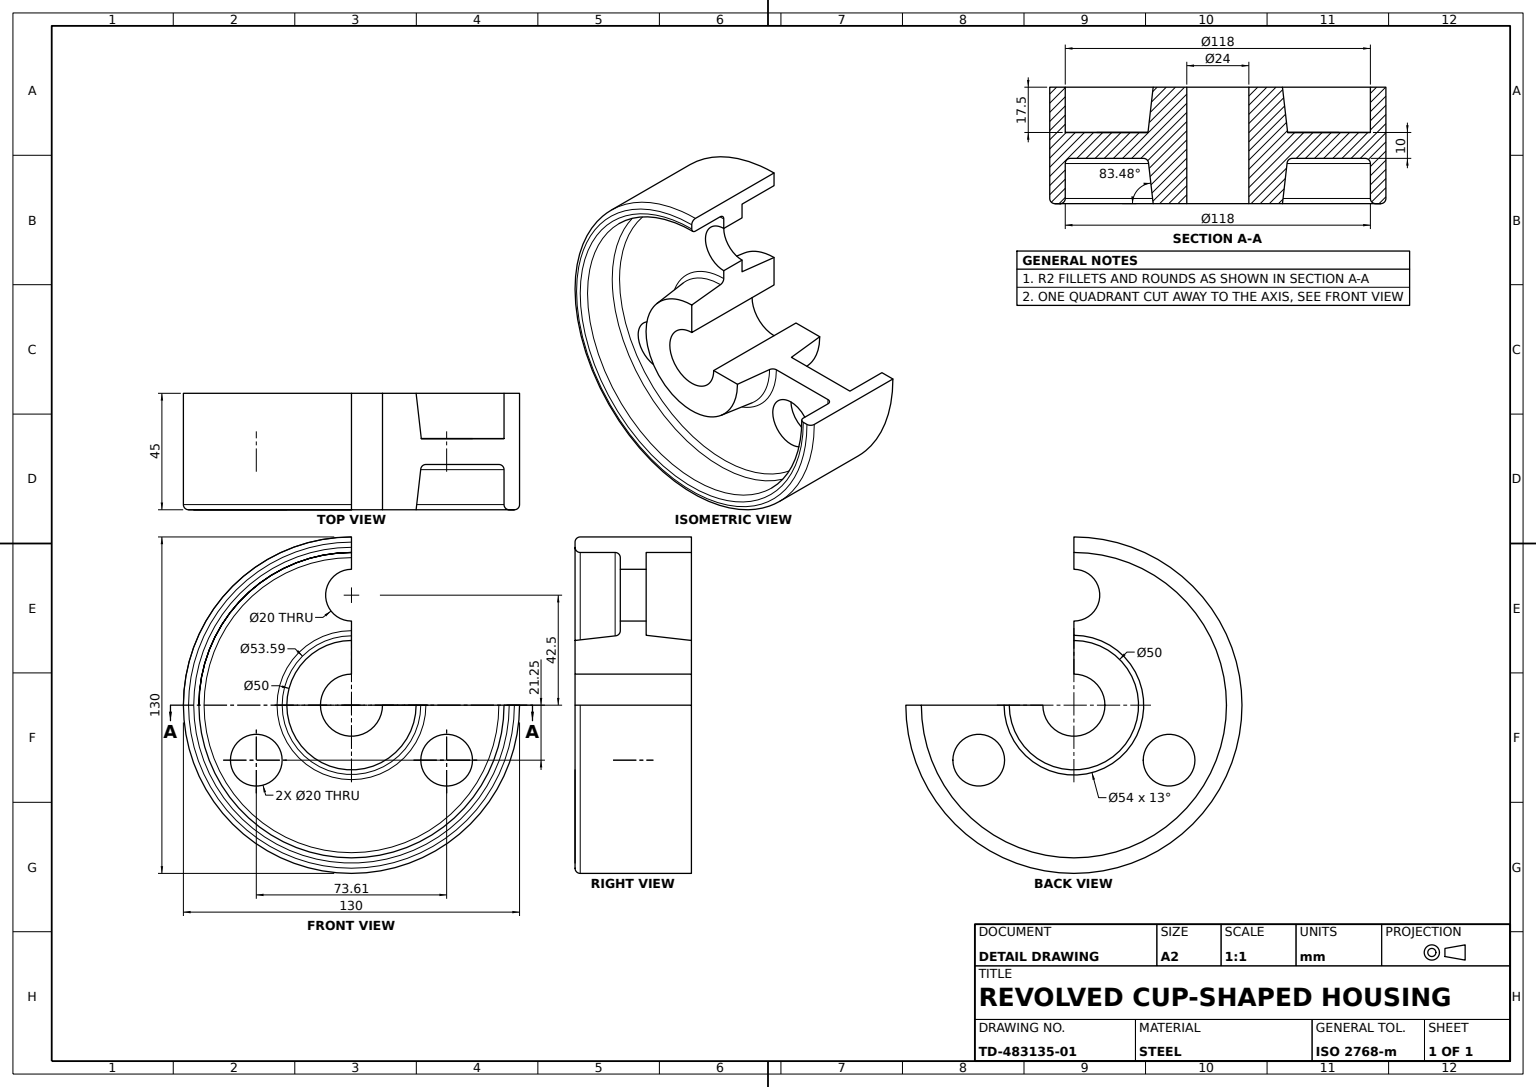
SolidWorks part; units mm, degrees
material "Plain Carbon Steel"
ref_plane "Front Plane" through (0, 0, 0) normal (0, 0, 1) x (1, 0, 0)
ref_plane "Top Plane" through (0, 0, 0) normal (0, 1, 0) x (1, 0, 0)
ref_plane "Right Plane" through (0, 0, 0) normal (1, 0, 0) x (0, 0, -1)
sketch "Wheel Profile Sketch" plane through (0, 0, 0) normal (0, 0, 1) x (1, 0, 0)
  line L0 (-53.0847, 0) -> (60.8825, 0)
  line L1 (0, 50.2951) -> (0, -47.8033) construction
  line L2 (0, 0) -> (0, 12)
  line L3 (22.5, 12) -> (-22.5, 12)
  line L4 (-22.5, 12) -> (-22.5, 25)
  line L5 (-22.5, 25) -> (-5, 27)
  line L6 (-5, 27) -> (-5, 59)
  line L7 (-5, 59) -> (-22.5, 59)
  line L8 (-22.5, 59) -> (-22.5, 65)
  line L9 (-22.5, 65) -> (22.5, 65)
  line L10 (22.5, 59) -> (22.5, 65)
  line L11 (5, 59) -> (22.5, 59)
  line L12 (5, 27) -> (5, 59)
  line L13 (22.5, 25) -> (5, 27)
  line L14 (22.5, 12) -> (22.5, 25)
  point P15 (0, 65)
  dimension "D1" = 12
  dimension "D2" = 22.5
  dimension "D3" = 13
  dimension "D4" = 15
  dimension "D5" = 6
  dimension "D6" = 5
  dimension "D7" = 53
  dimension "D8" = 17.5
  dimension "D9" = 53.0847
  dimension "D10" = 113.9672
revolve "Wheel Body Revolve" add sketch "Wheel Profile Sketch" angle 360 about L0
sketch "Rim Slot Sketch" plane through (5, 0, 0) normal (1, 0, 0) x (0, 0, -1)
  circle A0 centre (0, 0) radius 42.5 construction
  circle A1 centre (0, 42.5) radius 10
  circle A2 centre (36.8061, -21.25) radius 10
  circle A3 centre (-36.8061, -21.25) radius 10
  point P12 (0, 0)
  dimension "D1" = 85
  dimension "D2" = 20
  dimension "D4" = 63.75
  dimension "D3" = 3
extrude "Rim Slot Cut" cut sketch "Rim Slot Sketch" against normal through all contours A1 | A3 | A2
fillet "Edge Fillet R2 A" radius 2 3 edges at (5, 0, 59) (5, 0, 27) (22.5, 0, 65)
fillet "Edge Fillet R2 B" radius 2 1 edges at (22.5, 0, 59)
sketch "Web Relief Sketch" plane through (5, 0, 0) normal (1, 0, 0) x (0, 0, -1)
  line L0 (0, 77.9926) -> (0, 0)
  line L1 (0, 0) -> (85.2806, 0)
  arc A0 (0, 77.9926) -> (85.2806, 0) centre (13.9611, 7.6372) cw
  circle A1 centre (0, 42.5) radius 10 construction
  dimension "D1" = 71.7273
  dimension "D2" = 13.9611
  dimension "D3" = 85.2806
extrude "Web Relief Cut" cut sketch "Web Relief Sketch" against normal through all both and the other way through all
